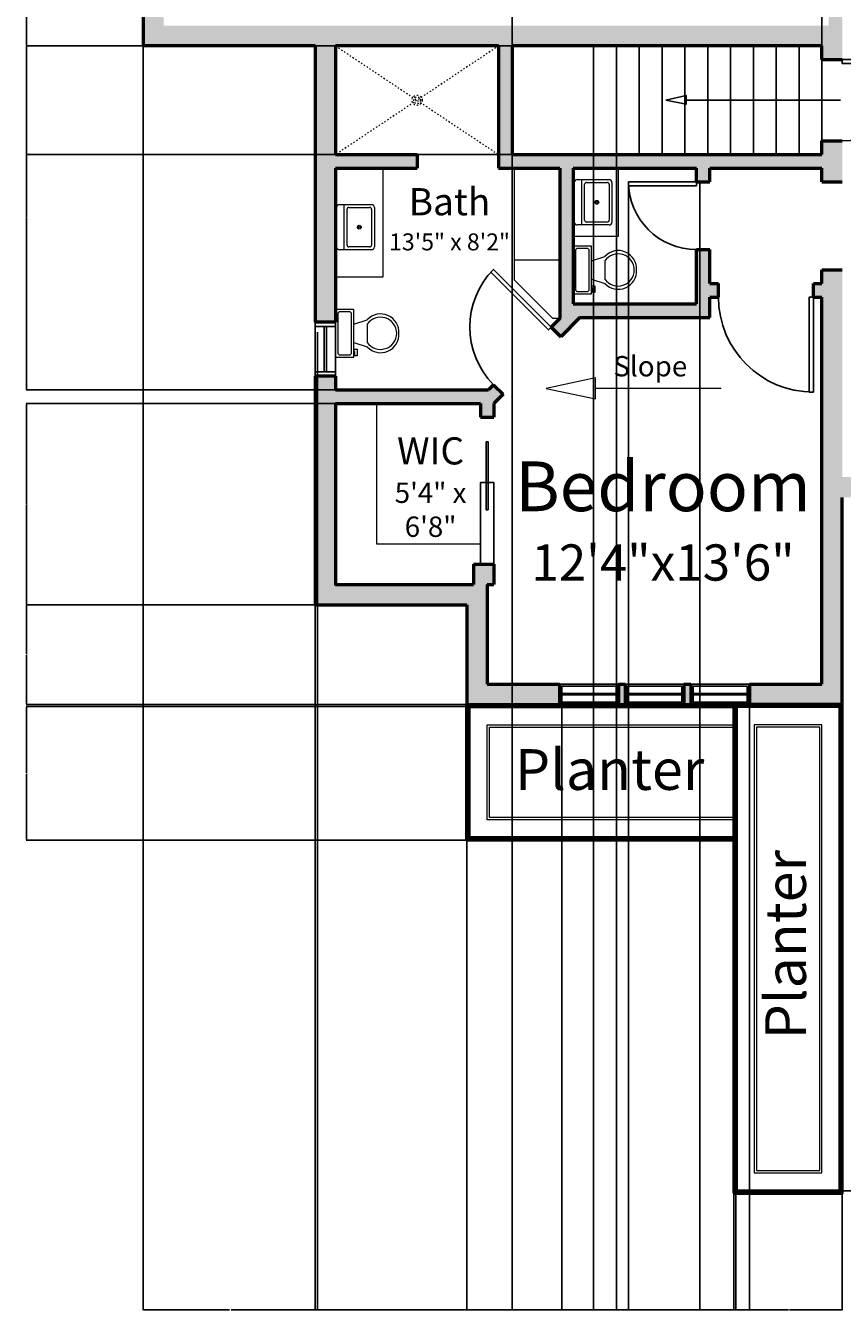
# Model space of a CAD drawing. Units: inches. Extents: x 296 to 2116, y 330 to 1460.
# Tile 1 of 9: x 296 to 657, y 330 to 898. Entities that reach past the tile are written whole.
import ezdxf

# ---------------------------------------------------------------- set-up
doc = ezdxf.new("R2010")
doc.units = ezdxf.units.IN
doc.linetypes.add('ACAD_ISO03W100', pattern=[30, 12, -18])
for name, color, linetype, lineweight in [('A-ANNO-DIMS', 2, 'Continuous', 18), ('A-ANNO-SYMB', 2, 'Continuous', 18), ('A-ANNO-TEXT', 7, 'Continuous', 18), ('A-AREA-IDEN', 7, 'Continuous', 25), ('A-DOOR', 3, 'Continuous', 25), ('A-FLOR-FIXT', 8, 'Continuous', 18), ('A-FLOR-OVHD', 132, 'ACAD_ISO03W100', 18), ('A-FLOR-STRS', 40, 'Continuous', 25), ('A-GLAZ', 4, 'Continuous', 25), ('A-WALL', 7, 'Continuous', 50), ('A-WALL-PATT', 8, 'Continuous', 13), ('L-PLNT', 90, 'Continuous', 18)]:
    doc.layers.add(name, color=color, linetype=linetype, lineweight=lineweight)
doc.styles.add('ATTR', font='romans.shx', dxfattribs={"width": 0.8, "height": 1.075})
doc.styles.get("Standard").update_dxf_attribs({"font": 'arial.ttf'})
doc.dimstyles.get("Standard").update_dxf_attribs({"dimtxt": 0.18, "dimasz": 0.18, "dimexe": 0.18, "dimexo": 0.0625, "dimgap": 0.09, "dimtad": 0, "dimtih": 1, "dimtoh": 1, "dimdec": 4, "dimzin": 0, "dimdsep": 46, "dimtxsty": 'Standard', "dimcen": 0.09, "dimadec": 0, "dimazin": 0, "dimtfac": 1, "dimtdec": 4, "dimtofl": 0, "dimtmove": 0, "dimatfit": 3, "dimfxl": 1, "dimtolj": 1, "dimtzin": 0, "dimarcsym": 0})

# ---------------------------------------------------------------- blocks, each defined once
blk = doc.blocks.new('*U2')
for p, q in [((0, 0), (0, -4)), ((-36, 0), (-36, -4))]:
    blk.add_line(p, q)
blk.add_lwpolyline([(0, 0), (0, 36), (-1.75, 36), (-1.75, 0)], close=True)
blk.add_arc((0, 0), 36, 90, 180)
blk = doc.blocks.new('*U4')
for p, q in [((-30, 0), (-30, -6)), ((0, 0), (0, -6))]:
    blk.add_line(p, q)
blk.add_lwpolyline([(0, 0), (0, 30), (-1.75, 30), (-1.75, 0)], close=True)
blk.add_arc((0, 0), 30, 90, 180)
blk = doc.blocks.new('*U3')
for p, q in [((0, 0), (0, -4)), ((40, 0), (40, -4))]:
    blk.add_line(p, q)
blk.add_lwpolyline([(0, 0), (0, 40), (1.75, 40), (1.75, 0)], close=True)
blk.add_arc((0, 0), 40, 0, 90)
blk = doc.blocks.new('*U15')
for p, q in [((-36, 0), (-36, 6)), ((0, 0), (0, 6))]:
    blk.add_line(p, q)
blk.add_lwpolyline([(0, 0), (0, -36), (-1.75, -36), (-1.75, 0)], close=True)
blk.add_arc((0, 0), 36, 180, 270)
blk = doc.blocks.new('*U29')
for p, q in [((9.5, -6), (9.5, -2)), ((-10, -8.5), (-8, -8.5)), ((-10, -9.5), (-10, -8.5)), ((-7, -9.5), (-10, -9.5)), ((-8, -8.5), (-8, -8)), ((-7, -8), (-7, -9.5)), ((-4, -8), (-6, -14)), ((4, -8), (6, -14)), ((4, -14), (-4, -14))]:
    blk.add_line(p, q)
blk.add_lwpolyline([(10.5, -8), (10.5, 0), (-10.5, 0), (-10.5, -8)], close=True)
for points in [[(-9.5, -2), (-9.5, -6)], [(8.5, -1), (-8.5, -1)], [(-8.5, -7), (8.5, -7)]]:
    blk.add_lwpolyline(points)
for centre, radius, start, end in [((-8.625, -1.875), 0.8839, 81.8699, 188.1301), ((8.625, -1.875), 0.8839, 351.8699, 98.1301), ((-8.625, -6.125), 0.8839, 171.869898, 278.1301), ((8.625, -6.125), 0.8839, 261.8699, 8.1301), ((-0.4772, -19.9188), 8.0953, 133.01722, 273.38), ((0.0374, -19.8731), 7.127, 124.50543, 269.7), ((-0.0373, -19.8731), 7.127, 270.3, 55.4946), ((0.4773, -19.9188), 8.0953, 266.62, 46.9828)]:
    blk.add_arc(centre, radius, start, end)
blk = doc.blocks.new("24'' Sink Single PV")
blk.add_line((-12.00001, -3.999996), (12, -3.999996))
for points in [[(-10.5, 0), (10.5, 0)], [(-12.00001, -18.499996), (-12.00001, -1.5)], [(-10.5, -17.499996), (-10.5, -6.499996)], [(-9.5, -5.499996), (9.5, -5.499996)], [(10.5, -6.499996), (10.5, -17.499996)], [(12, -1.5), (12, -18.499996)], [(10.5, -19.999996), (-10.5, -19.999996)], [(9.5, -18.499996), (-9.5, -18.499996)]]:
    blk.add_lwpolyline(points)
for radius in [1, 0.5]:
    blk.add_circle((0, -11.999996), radius)
for centre, radius, start, end in [((-10.5, -1.5), 1.5, 90, 180), ((-9.5, -6.499996), 1, 90, 180), ((9.5, -6.499996), 1, 0, 90), ((10.5, -1.5), 1.5, 0, 90), ((-10.5, -18.499996), 1.5, 180, 270), ((-9.5, -17.499996), 1, 180, 270), ((9.5, -17.499996), 1, 270, 0), ((10.5, -18.499996), 1.5, 270, 0)]:
    blk.add_arc(centre, radius, start, end)
at = {"style": 'ATTR', "width": 0.8, "flags": 9}
blk.add_attdef('ESTCODE', (0, 0), '', height=0.0048, dxfattribs=at)
blk = doc.blocks.new('SLOPE-ARROW')
blk.add_line((739.99, 662.71), (684.54, 662.71))
blk.add_lwpolyline([(662.67, 662.71), (684.54, 658.1), (684.54, 667.32)], close=True)
blk = doc.blocks.new('*D45')
at = {"layer": 'A-ANNO-DIMS', "color": 0, "lineweight": -2, "transparency": 16777216}
for p, q in [((1156.58, 1407.95), (1235.3, 1407.95)), ((1235.12, 1407.77), (1235.12, 895.66)), ((1235.12, 383.18), (1235.12, 895.29)), ((609.63, 383), (1235.3, 383))]:
    blk.add_line(p, q, dxfattribs=at)
at = {"layer": 'A-ANNO-DIMS', "color": 0, "transparency": 16777216}
for points in [[(1235.09, 1407.77), (1235.15, 1407.77), (1235.12, 1407.95)], [(1235.09, 383.18), (1235.15, 383.18), (1235.12, 383)]]:
    blk.add_solid(points, dxfattribs=at)
at = {"layer": 'Defpoints', "color": 0, "transparency": 16777216}
for p in [(1156.52, 1407.95), (1235.12, 1407.95), (609.57, 383)]:
    blk.add_point(p, dxfattribs=at)
at = {"layer": 'A-ANNO-DIMS', "color": 0, "transparency": 16777216, "insert": (1235.12, 895.48), "char_height": 0.18, "attachment_point": 5}
blk.add_mtext('\\A1;1025', dxfattribs=at)
blk = doc.blocks.new('*D50')
at = {"layer": 'A-ANNO-DIMS', "color": 0, "lineweight": -2, "transparency": 16777216}
for p, q in [((347.52, 888.94), (347.52, 330.22)), ((424.57, 762.44), (424.57, 330.22)), ((347.7, 330.4), (385.65, 330.4)), ((424.39, 330.4), (386.44, 330.4))]:
    blk.add_line(p, q, dxfattribs=at)
at = {"layer": 'A-ANNO-DIMS', "color": 0, "transparency": 16777216}
for points in [[(347.7, 330.43), (347.7, 330.37), (347.52, 330.4)], [(424.39, 330.43), (424.39, 330.37), (424.57, 330.4)]]:
    blk.add_solid(points, dxfattribs=at)
at = {"layer": 'Defpoints', "color": 0, "transparency": 16777216}
for p in [(347.52, 889), (424.57, 762.5), (424.57, 330.4)]:
    blk.add_point(p, dxfattribs=at)
at = {"layer": 'A-ANNO-DIMS', "color": 0, "transparency": 16777216, "insert": (386.05, 330.4), "char_height": 0.18, "attachment_point": 5}
blk.add_mtext('\\A1;77.05', dxfattribs=at)
blk = doc.blocks.new('*D51')
at = {"layer": 'A-ANNO-DIMS', "color": 0, "lineweight": -2, "transparency": 16777216}
for p, q in [((424.57, 762.44), (424.57, 330.22)), ((490.57, 537.98), (490.57, 330.22)), ((424.75, 330.4), (457.35, 330.4)), ((490.39, 330.4), (457.79, 330.4))]:
    blk.add_line(p, q, dxfattribs=at)
at = {"layer": 'A-ANNO-DIMS', "color": 0, "transparency": 16777216}
for points in [[(424.75, 330.43), (424.75, 330.37), (424.57, 330.4)], [(490.39, 330.43), (490.39, 330.37), (490.57, 330.4)]]:
    blk.add_solid(points, dxfattribs=at)
at = {"layer": 'Defpoints', "color": 0, "transparency": 16777216}
for p in [(424.57, 762.5), (490.57, 538.04), (490.57, 330.4)]:
    blk.add_point(p, dxfattribs=at)
at = {"layer": 'A-ANNO-DIMS', "color": 0, "transparency": 16777216, "insert": (457.57, 330.4), "char_height": 0.18, "attachment_point": 5}
blk.add_mtext('\\A1;66', dxfattribs=at)
blk = doc.blocks.new('*D52')
at = {"layer": 'A-ANNO-DIMS', "color": 0, "lineweight": -2, "transparency": 16777216}
for p, q in [((490.57, 537.98), (490.57, 330.22)), ((608.57, 537.98), (608.57, 330.22)), ((490.75, 330.4), (549.29, 330.4)), ((608.39, 330.4), (549.85, 330.4))]:
    blk.add_line(p, q, dxfattribs=at)
at = {"layer": 'A-ANNO-DIMS', "color": 0, "transparency": 16777216}
for points in [[(490.75, 330.43), (490.75, 330.37), (490.57, 330.4)], [(608.39, 330.43), (608.39, 330.37), (608.57, 330.4)]]:
    blk.add_solid(points, dxfattribs=at)
at = {"layer": 'Defpoints', "color": 0, "transparency": 16777216}
for p in [(490.57, 538.04), (608.57, 538.04), (608.57, 330.4)]:
    blk.add_point(p, dxfattribs=at)
at = {"layer": 'A-ANNO-DIMS', "color": 0, "transparency": 16777216, "insert": (549.57, 330.4), "char_height": 0.18, "attachment_point": 5}
blk.add_mtext('\\A1;118', dxfattribs=at)
blk = doc.blocks.new('*D53')
at = {"layer": 'A-ANNO-DIMS', "color": 0, "lineweight": -2, "transparency": 16777216}
for p, q in [((609.57, 382.94), (609.57, 330.22)), ((656.57, 381.94), (656.57, 330.22)), ((609.75, 330.4), (632.85, 330.4)), ((656.39, 330.4), (633.29, 330.4))]:
    blk.add_line(p, q, dxfattribs=at)
at = {"layer": 'A-ANNO-DIMS', "color": 0, "transparency": 16777216}
for points in [[(609.75, 330.43), (609.75, 330.37), (609.57, 330.4)], [(656.39, 330.43), (656.39, 330.37), (656.57, 330.4)]]:
    blk.add_solid(points, dxfattribs=at)
at = {"layer": 'Defpoints', "color": 0, "transparency": 16777216}
for p in [(609.57, 383), (656.57, 382), (656.57, 330.4)]:
    blk.add_point(p, dxfattribs=at)
at = {"layer": 'A-ANNO-DIMS', "color": 0, "transparency": 16777216, "insert": (633.07, 330.4), "char_height": 0.18, "attachment_point": 5}
blk.add_mtext('\\A1;47', dxfattribs=at)
blk = doc.blocks.new('*D57')
at = {"layer": 'A-ANNO-DIMS', "color": 0, "lineweight": -2, "transparency": 16777216}
for p, q in [((491.51, 597), (295.74, 597)), ((295.92, 596.82), (295.92, 567.7)), ((295.92, 538.22), (295.92, 567.34)), ((490.51, 538.04), (295.74, 538.04))]:
    blk.add_line(p, q, dxfattribs=at)
at = {"layer": 'A-ANNO-DIMS', "color": 0, "transparency": 16777216}
for points in [[(295.89, 596.82), (295.95, 596.82), (295.92, 597)], [(295.89, 538.22), (295.95, 538.22), (295.92, 538.04)]]:
    blk.add_solid(points, dxfattribs=at)
at = {"layer": 'Defpoints', "color": 0, "transparency": 16777216}
for p in [(295.92, 597), (491.57, 597), (490.57, 538.04)]:
    blk.add_point(p, dxfattribs=at)
at = {"layer": 'A-ANNO-DIMS', "color": 0, "transparency": 16777216, "insert": (295.92, 567.52), "char_height": 0.18, "attachment_point": 5}
blk.add_mtext('\\A1;58.96', dxfattribs=at)
blk = doc.blocks.new('*D58')
at = {"layer": 'A-ANNO-DIMS', "color": 0, "lineweight": -2, "transparency": 16777216}
for p, q in [((347.46, 1031), (295.74, 1031)), ((295.92, 1030.82), (295.92, 960.18)), ((295.92, 889.18), (295.92, 959.82)), ((347.46, 889), (295.74, 889))]:
    blk.add_line(p, q, dxfattribs=at)
at = {"layer": 'A-ANNO-DIMS', "color": 0, "transparency": 16777216}
for points in [[(295.89, 1030.82), (295.95, 1030.82), (295.92, 1031)], [(295.89, 889.18), (295.95, 889.18), (295.92, 889)]]:
    blk.add_solid(points, dxfattribs=at)
at = {"layer": 'Defpoints', "color": 0, "transparency": 16777216}
for p in [(295.92, 1031), (347.52, 1031), (347.52, 889)]:
    blk.add_point(p, dxfattribs=at)
at = {"layer": 'A-ANNO-DIMS', "color": 0, "transparency": 16777216, "insert": (295.92, 960), "char_height": 0.18, "attachment_point": 5}
blk.add_mtext('\\A1;142', dxfattribs=at)
blk = doc.blocks.new('*D66')
at = {"layer": 'A-ANNO-DIMS', "color": 0, "lineweight": -2, "transparency": 16777216}
for p, q in [((510.57, 889.06), (510.57, 1459.73)), ((510.75, 1459.55), (578.79, 1459.55)), ((647.39, 1459.55), (579.35, 1459.55)), ((647.57, 889.06), (647.57, 1459.73))]:
    blk.add_line(p, q, dxfattribs=at)
at = {"layer": 'A-ANNO-DIMS', "color": 0, "transparency": 16777216}
for points in [[(510.75, 1459.58), (510.75, 1459.52), (510.57, 1459.55)], [(647.39, 1459.58), (647.39, 1459.52), (647.57, 1459.55)]]:
    blk.add_solid(points, dxfattribs=at)
at = {"layer": 'Defpoints', "color": 0, "transparency": 16777216}
for p in [(647.57, 1459.55), (510.57, 889), (647.57, 889)]:
    blk.add_point(p, dxfattribs=at)
at = {"layer": 'A-ANNO-DIMS', "color": 0, "transparency": 16777216, "insert": (579.07, 1459.55), "char_height": 0.18, "attachment_point": 5}
blk.add_mtext('\\A1;137', dxfattribs=at)
blk = doc.blocks.new('*D89')
at = {"layer": 'A-ANNO-DIMS', "color": 0, "lineweight": -2, "transparency": 16777216}
for p, q in [((423.57, 888.94), (423.57, 330.22)), ((510.57, 888.94), (510.57, 330.22)), ((423.75, 330.4), (466.68, 330.4)), ((510.39, 330.4), (467.47, 330.4))]:
    blk.add_line(p, q, dxfattribs=at)
at = {"layer": 'A-ANNO-DIMS', "color": 0, "transparency": 16777216}
for points in [[(423.75, 330.43), (423.75, 330.37), (423.57, 330.4)], [(510.39, 330.43), (510.39, 330.37), (510.57, 330.4)]]:
    blk.add_solid(points, dxfattribs=at)
at = {"layer": 'Defpoints', "color": 0, "transparency": 16777216}
for p in [(423.57, 889), (510.57, 889), (510.57, 330.4)]:
    blk.add_point(p, dxfattribs=at)
at = {"layer": 'A-ANNO-DIMS', "color": 0, "transparency": 16777216, "insert": (467.07, 330.4), "char_height": 0.18, "attachment_point": 5}
blk.add_mtext('\\A1;87.00', dxfattribs=at)
blk = doc.blocks.new('*D90')
at = {"layer": 'A-ANNO-DIMS', "color": 0, "lineweight": -2, "transparency": 16777216}
for p, q in [((546.57, 840.94), (546.57, 330.22)), ((556.67, 840.94), (556.67, 330.22)), ((546.75, 330.4), (551.24, 330.4)), ((556.49, 330.4), (552.01, 330.4))]:
    blk.add_line(p, q, dxfattribs=at)
at = {"layer": 'A-ANNO-DIMS', "color": 0, "transparency": 16777216}
for points in [[(546.75, 330.43), (546.75, 330.37), (546.57, 330.4)], [(556.49, 330.43), (556.49, 330.37), (556.67, 330.4)]]:
    blk.add_solid(points, dxfattribs=at)
at = {"layer": 'Defpoints', "color": 0, "transparency": 16777216}
for p in [(546.57, 841), (556.67, 841), (556.67, 330.4)]:
    blk.add_point(p, dxfattribs=at)
at = {"layer": 'A-ANNO-DIMS', "color": 0, "transparency": 16777216, "insert": (551.62, 330.4), "char_height": 0.18, "attachment_point": 5}
blk.add_mtext('\\A1;10.10', dxfattribs=at)
blk = doc.blocks.new('*D91')
at = {"layer": 'A-ANNO-DIMS', "color": 0, "lineweight": -2, "transparency": 16777216}
for p, q in [((597.01, 889), (295.74, 889)), ((295.92, 888.82), (295.92, 865.18)), ((295.92, 841.18), (295.92, 864.82)), ((597.01, 841), (295.74, 841))]:
    blk.add_line(p, q, dxfattribs=at)
at = {"layer": 'A-ANNO-DIMS', "color": 0, "transparency": 16777216}
for points in [[(295.89, 888.82), (295.95, 888.82), (295.92, 889)], [(295.89, 841.18), (295.95, 841.18), (295.92, 841)]]:
    blk.add_solid(points, dxfattribs=at)
at = {"layer": 'Defpoints', "color": 0, "transparency": 16777216}
for p in [(597.07, 889), (295.92, 841), (597.07, 841)]:
    blk.add_point(p, dxfattribs=at)
at = {"layer": 'A-ANNO-DIMS', "color": 0, "transparency": 16777216, "insert": (295.92, 865), "char_height": 0.18, "attachment_point": 5}
blk.add_mtext('\\A1;48.00', dxfattribs=at)
blk = doc.blocks.new('*D92')
at = {"layer": 'A-ANNO-DIMS', "color": 0, "lineweight": -2, "transparency": 16777216}
for p, q in [((432.51, 731), (295.74, 731)), ((295.92, 730.82), (295.92, 686.68)), ((295.92, 642.18), (295.92, 686.32)), ((423.51, 642), (295.74, 642))]:
    blk.add_line(p, q, dxfattribs=at)
at = {"layer": 'A-ANNO-DIMS', "color": 0, "transparency": 16777216}
for points in [[(295.89, 730.82), (295.95, 730.82), (295.92, 731)], [(295.89, 642.18), (295.95, 642.18), (295.92, 642)]]:
    blk.add_solid(points, dxfattribs=at)
at = {"layer": 'Defpoints', "color": 0, "transparency": 16777216}
for p in [(432.57, 731), (295.92, 642), (423.57, 642)]:
    blk.add_point(p, dxfattribs=at)
at = {"layer": 'A-ANNO-DIMS', "color": 0, "transparency": 16777216, "insert": (295.92, 686.5), "char_height": 0.18, "attachment_point": 5}
blk.add_mtext('\\A1;89.00', dxfattribs=at)
blk = doc.blocks.new('*D93')
at = {"layer": 'A-ANNO-DIMS', "color": 0, "lineweight": -2, "transparency": 16777216}
for p, q in [((423.51, 889), (295.74, 889)), ((295.92, 888.82), (295.92, 813.18)), ((295.92, 737.18), (295.92, 812.82)), ((432.51, 737), (295.74, 737))]:
    blk.add_line(p, q, dxfattribs=at)
at = {"layer": 'A-ANNO-DIMS', "color": 0, "transparency": 16777216}
for points in [[(295.89, 888.82), (295.95, 888.82), (295.92, 889)], [(295.89, 737.18), (295.95, 737.18), (295.92, 737)]]:
    blk.add_solid(points, dxfattribs=at)
at = {"layer": 'Defpoints', "color": 0, "transparency": 16777216}
for p in [(295.92, 889), (423.57, 889), (432.57, 737)]:
    blk.add_point(p, dxfattribs=at)
at = {"layer": 'A-ANNO-DIMS', "color": 0, "transparency": 16777216, "insert": (295.92, 813), "char_height": 0.18, "attachment_point": 5}
blk.add_mtext('\\A1;152.00', dxfattribs=at)
blk = doc.blocks.new('*D94')
at = {"layer": 'A-ANNO-DIMS', "color": 0, "lineweight": -2, "transparency": 16777216}
for p, q in [((423.51, 642), (295.74, 642)), ((295.92, 641.82), (295.92, 620.18)), ((295.92, 598.18), (295.92, 619.82)), ((490.51, 598), (295.74, 598))]:
    blk.add_line(p, q, dxfattribs=at)
at = {"layer": 'A-ANNO-DIMS', "color": 0, "transparency": 16777216}
for points in [[(295.89, 641.82), (295.95, 641.82), (295.92, 642)], [(295.89, 598.18), (295.95, 598.18), (295.92, 598)]]:
    blk.add_solid(points, dxfattribs=at)
at = {"layer": 'Defpoints', "color": 0, "transparency": 16777216}
for p in [(295.92, 642), (423.57, 642), (490.57, 598)]:
    blk.add_point(p, dxfattribs=at)
at = {"layer": 'A-ANNO-DIMS', "color": 0, "transparency": 16777216, "insert": (295.92, 620), "char_height": 0.18, "attachment_point": 5}
blk.add_mtext('\\A1;44.00', dxfattribs=at)
blk = doc.blocks.new('*D102')
at = {"layer": 'A-ANNO-DIMS', "color": 0, "lineweight": -2, "transparency": 16777216}
for p, q in [((562.07, 828.94), (562.07, 330.22)), ((593.59, 828.06), (593.59, 330.22)), ((562.25, 330.4), (577.37, 330.4)), ((593.41, 330.4), (578.29, 330.4))]:
    blk.add_line(p, q, dxfattribs=at)
at = {"layer": 'A-ANNO-DIMS', "color": 0, "transparency": 16777216}
for points in [[(562.25, 330.43), (562.25, 330.37), (562.07, 330.4)], [(593.41, 330.43), (593.41, 330.37), (593.59, 330.4)]]:
    blk.add_solid(points, dxfattribs=at)
at = {"layer": 'Defpoints', "color": 0, "transparency": 16777216}
for p in [(562.07, 829), (593.59, 828.12), (593.59, 330.4)]:
    blk.add_point(p, dxfattribs=at)
at = {"layer": 'A-ANNO-DIMS', "color": 0, "transparency": 16777216, "insert": (577.83, 330.4), "char_height": 0.18, "attachment_point": 5}
blk.add_mtext('\\A1;31.516', dxfattribs=at)
blk = doc.blocks.new('*D105')
at = {"layer": 'A-ANNO-DIMS', "color": 0, "lineweight": -2, "transparency": 16777216}
for p, q in [((532.57, 598.94), (532.57, 330.22)), ((615.57, 597.94), (615.57, 330.22)), ((532.75, 330.4), (573.68, 330.4)), ((615.39, 330.4), (574.47, 330.4))]:
    blk.add_line(p, q, dxfattribs=at)
at = {"layer": 'A-ANNO-DIMS', "color": 0, "transparency": 16777216}
for points in [[(532.75, 330.43), (532.75, 330.37), (532.57, 330.4)], [(615.39, 330.43), (615.39, 330.37), (615.57, 330.4)]]:
    blk.add_solid(points, dxfattribs=at)
at = {"layer": 'Defpoints', "color": 0, "transparency": 16777216}
for p in [(532.57, 599), (615.57, 598), (615.57, 330.4)]:
    blk.add_point(p, dxfattribs=at)
at = {"layer": 'A-ANNO-DIMS', "color": 0, "transparency": 16777216, "insert": (574.07, 330.4), "char_height": 0.18, "attachment_point": 5}
blk.add_mtext('\\A1;83.00', dxfattribs=at)

msp = doc.modelspace()

# ---------------------------------------------------------------- hatches: boundary and pattern name
at = {"layer": 'A-WALL-PATT'}
h = msp.add_hatch(color=256, dxfattribs=at)
h.dxf.hatch_style = 1
h.paths.add_polyline_path([(656.5723, 927.9991), (668.5723, 927.9991), (668.5723, 936.9991), (650.5723, 936.9991), (650.5723, 897.9991), (356.5223, 897.9991), (356.5223, 955.9991), (347.5223, 955.9991), (347.5223, 888.9991), (423.5723, 888.9991), (423.5723, 766.9991), (432.5723, 766.9991), (432.5723, 834.9991), (453.5723, 834.9991), (468.5723, 834.9991), (468.5723, 840.9991), (432.5723, 840.9991), (432.5723, 888.9991), (504.5723, 888.9991), (504.5723, 840.9991), (504.5723, 834.9991), (531.6223, 834.9991), (531.6223, 768.5344), (527.8443, 764.7564), (530.6728, 761.928), (532.087, 760.5138), (540.5723, 768.9991), (598.0723, 768.9991), (598.0723, 777.9991), (601.8223, 777.9991), (601.8223, 782.1991), (601.8223, 783.9991), (598.0723, 783.9991), (598.0723, 798.9991), (592.0723, 798.9991), (592.0723, 774.9991), (537.6223, 774.9991), (537.6223, 834.9991), (592.0723, 834.9991), (592.0723, 828.9991), (598.0723, 828.9991), (598.0723, 834.9991), (647.5723, 834.9991), (647.5723, 828.9991), (656.5723, 828.9991), (656.5723, 846.9991), (650.5723, 846.9991), (647.5723, 846.9991), (647.5723, 840.9991), (510.5723, 840.9991), (510.5723, 888.9991), (647.5723, 888.9991), (647.5723, 882.9991), (656.5723, 882.9991)])
h.paths.add_polyline_path([(432.5723, 730.9991), (496.5723, 730.9991), (496.5723, 724.9991), (502.5723, 724.9991), (502.5723, 730.9991), (506.6311, 735.058), (502.3885, 739.3006), (500.087, 736.9991), (432.5723, 736.9991), (432.5723, 742.9991), (423.5723, 742.9991), (423.5723, 641.9991), (490.5723, 641.9991), (490.5723, 597.9991), (531.5723, 597.9991), (531.5723, 606.9991), (499.5723, 606.9991), (499.5723, 650.9991), (502.5723, 650.9991), (502.5723, 659.9991), (496.5723, 659.9991), (493.5723, 659.9991), (493.5723, 650.9991), (432.5723, 650.9991)])
h.paths.add_polyline_path([(656.5723, 689.4991), (662.5473, 689.4991), (662.5473, 698.4991), (656.5723, 698.4991), (656.5723, 789.9991), (647.5723, 789.9991), (647.5723, 783.9991), (643.8223, 783.9991), (643.8223, 777.9991), (647.5723, 777.9991), (647.5723, 606.9991), (615.5723, 606.9991), (615.5723, 597.9991), (656.5723, 597.9991)])
h.paths.add_polyline_path([(761.5223, 780.9541), (797.5223, 780.9541), (797.5223, 789.9541), (761.5223, 789.9541), (761.5223, 858.9541), (797.5223, 858.9541), (797.5223, 867.9541), (752.5223, 867.9541), (752.5223, 698.4991), (746.5473, 698.4991), (746.5473, 694.2991), (746.5473, 689.4991), (752.5223, 689.4991), (752.5223, 624.9541), (761.5223, 624.9541)])
h.paths.add_polyline_path([(1102.5223, 795.9541), (1093.5223, 795.9541), (1093.5223, 789.9541), (1063.5223, 789.9541), (881.5223, 789.9541), (881.5223, 837.9541), (911.5223, 837.9541), (911.5223, 849.9541), (907.5223, 849.9541), (905.5223, 849.9541), (905.5223, 843.9541), (845.5223, 843.9541), (845.5223, 834.9541), (849.0223, 834.9541), (851.5223, 834.9541), (851.5223, 837.9541), (875.5223, 837.9541), (875.5223, 789.9541), (851.5223, 789.9541), (851.5223, 792.9541), (845.5223, 792.9541), (845.5223, 789.9541), (833.5223, 789.9541), (833.5223, 785.1541), (833.5223, 780.9541), (1049.5223, 780.9541), (1049.5223, 726.9541), (1053.7223, 726.9541), (1058.5223, 726.9541), (1058.5223, 780.9541), (1102.5223, 780.9541)])
h.paths.add_polyline_path([(761.5223, 588.9541), (752.5223, 588.9541), (752.5223, 564.9541), (761.5223, 564.9541)])
h.paths.add_polyline_path([(809.5223, 480.9541), (761.5223, 480.9541), (761.5223, 528.9541), (752.5223, 528.9541), (752.5223, 471.9541), (809.5223, 471.9541)])
h.paths.add_polyline_path([(1058.5223, 684.9541), (1049.5223, 684.9541), (1049.5223, 480.9541), (1001.5223, 480.9541), (1001.5223, 476.4541), (1001.5223, 471.9541), (1058.5223, 471.9541)])
h.paths.add_polyline_path([(794.5223, 1013.9991), (800.5223, 1013.9991), (800.5223, 1019.9991), (794.5223, 1019.9991), (794.5223, 1296.9541), (785.5223, 1296.9541), (785.5223, 1221.9991), (752.5223, 1221.9991), (752.5223, 1212.9991), (788.5223, 1212.9991), (788.5223, 936.9991), (752.5223, 936.9991), (752.5223, 927.9991), (794.5223, 927.9991)])
h.paths.add_polyline_path([(450.0223, 1191.9991), (398.5223, 1191.9991), (398.5223, 1137.9991), (407.5223, 1137.9991), (407.5223, 1182.9991), (450.0223, 1182.9991)])
h.paths.add_polyline_path([(576.5223, 1212.9991), (612.5223, 1212.9991), (612.5223, 1221.9991), (567.5223, 1221.9991), (567.5223, 1191.9991), (540.0223, 1191.9991), (540.0223, 1182.9991), (576.5223, 1182.9991)])
h.paths.add_polyline_path([(407.5223, 1060.9991), (398.5223, 1060.9991), (398.5223, 1030.9991), (392.5223, 1030.9991), (392.5223, 1021.9991), (407.5223, 1021.9991)])
h.paths.add_polyline_path([(356.5223, 1030.9991), (347.5223, 1030.9991), (347.5223, 1015.9991), (356.5223, 1015.9991), (356.5223, 1021.9991)])
h.paths.add_polyline_path([(788.5223, 1129.9991), (770.0334, 1131.3572, 0.43585667), (767.8869, 1129.3626), (767.8869, 1108.3618, 0.31855172), (769.8942, 1105.5308), (788.5223, 1098.9991)], flags=17)
h.paths.add_polyline_path([(788.5223, 1050.9991), (769.8942, 1044.4674, 0.31855172), (767.8869, 1041.6364), (767.8869, 1020.6356, 0.43585667), (770.0334, 1018.641), (788.5223, 1019.9991)], flags=17)
h.paths.add_polyline_path([(893.5223, 1066.9541), (851.5223, 1066.9541), (851.5223, 1069.9541), (845.5223, 1069.9541), (845.5223, 1019.9991), (839.5223, 1019.9991), (839.5223, 1013.9991), (845.5223, 1013.9991), (845.5223, 891.9541), (863.5223, 891.9541), (863.5223, 897.9541), (851.5223, 897.9541), (851.5223, 927.9541), (905.5223, 927.9541), (905.5223, 897.9541), (893.5223, 897.9541), (893.5223, 891.9541), (905.5223, 891.9541), (905.5223, 885.9541), (911.5223, 885.9541), (911.5223, 927.9541), (1030.5223, 927.9541), (1030.5223, 936.9541), (1013.5223, 936.9541), (1013.5223, 996.9541), (1093.5223, 996.9541), (1093.5223, 936.9541), (1066.5223, 936.9541), (1066.5223, 927.9541), (1093.5223, 927.9541), (1093.5223, 921.9541), (1102.5223, 921.9541), (1102.5223, 1013.9541), (1093.5223, 1013.9541), (1093.5223, 1002.9541), (1013.5223, 1002.9541), (1013.5223, 1060.9541), (1013.5223, 1066.9541), (1007.5223, 1066.9541), (1007.5223, 1042.9541), (977.5223, 1042.9541), (977.5223, 1066.9541), (965.5223, 1066.9541), (965.5223, 1060.9541), (971.5223, 1060.9541), (971.5223, 1036.9541), (1007.5223, 1036.9541), (1007.5223, 936.9541), (851.5223, 936.9541), (851.5223, 1060.9541), (893.5223, 1060.9541)])
h.paths.add_polyline_path([(851.5223, 1150.9541), (919.5223, 1150.9541), (919.5223, 1114.9541), (911.5223, 1114.9541), (911.5223, 1108.9541), (925.5223, 1108.9541), (925.5223, 1150.9541), (1007.5223, 1150.9541), (1007.5223, 1114.9541), (1013.5223, 1114.9541), (1013.5223, 1150.9541), (1046.5223, 1150.9541), (1046.5223, 1159.9541), (1007.5223, 1159.9541), (1007.5223, 1186.9541), (998.5223, 1186.9541), (998.5223, 1156.9541), (845.5223, 1156.9541), (845.5223, 1105.9541), (851.5223, 1105.9541)])
h.paths.add_polyline_path([(1102.5223, 1156.9541), (1102.5223, 1159.9541), (1088.5223, 1159.9541), (1088.5223, 1150.9541), (1093.5223, 1150.9541), (1093.5223, 1147.9541), (1102.5223, 1147.9541)])
h.paths.add_polyline_path([(1102.5223, 1111.9541), (1093.5223, 1111.9541), (1093.5223, 1066.9541), (1047.5223, 1066.9541), (1047.5223, 1030.9541), (1053.5223, 1030.9541), (1053.5223, 1060.9541), (1093.5223, 1060.9541), (1093.5223, 1049.9541), (1102.5223, 1049.9541)])
h.paths.add_polyline_path([(1102.5223, 837.9541), (1093.5223, 837.9541), (1093.5223, 831.9541), (1102.5223, 831.9541)], flags=17)
h.paths.add_polyline_path([(1102.5223, 879.9541), (1093.5223, 879.9541), (1093.5223, 873.9541), (1102.5223, 873.9541)])
h.paths.add_polyline_path([(839.5223, 1353.9541), (785.5223, 1353.9541), (785.5223, 1338.9541), (794.5223, 1338.9541), (794.5223, 1344.9541), (839.5223, 1344.9541)])
h.paths.add_polyline_path([(1007.5223, 1353.9541), (953.5223, 1353.9541), (953.5223, 1344.9541), (998.5223, 1344.9541), (998.5223, 1314.9541), (1007.5223, 1314.9541)])
h.paths.add_polyline_path([(917.5223, 1353.9541), (914.5223, 1353.9541), (914.5223, 1344.9541), (917.5223, 1344.9541)])
h.paths.add_polyline_path([(878.5223, 1353.9541), (875.5223, 1353.9541), (875.5223, 1344.9541), (878.5223, 1344.9541)])
h.paths.add_polyline_path([(1007.5223, 1278.9541), (998.5223, 1278.9541), (998.5223, 1222.9541), (1007.5223, 1222.9541)])
h.paths.add_polyline_path([(407.5223, 1101.9991), (398.5223, 1101.9991), (398.5223, 1096.9991), (407.5223, 1096.9991)])
h.paths.add_polyline_path([(560.5723, 606.9991), (557.5723, 606.9991), (557.5723, 597.9991), (560.5723, 597.9991)])
h.paths.add_polyline_path([(589.5723, 606.9991), (586.5723, 606.9991), (586.5723, 597.9991), (589.5723, 597.9991)])

# ---------------------------------------------------------------- linework, layer by layer
at = {"layer": 'A-DOOR'}
for points in [[(500.0723, 683.9991), (500.0723, 713.9991), (499.0723, 713.9991), (499.0723, 683.9991)], [(496.5723, 659.9991), (496.5723, 695.9991), (502.5723, 695.9991), (502.5723, 659.9991)]]:
    msp.add_lwpolyline(points, close=True, dxfattribs=at)
at = {"layer": 'A-FLOR-FIXT'}
for p, q in [((511.6517, 785.5049), (511.6517, 834.9991)), ((557.6223, 804.9991), (557.6223, 834.9991)), ((537.6223, 804.9991), (557.6223, 804.9991)), ((511.6517, 794.5049), (531.6223, 794.5049)), ((528.6223, 768.5344), (511.6517, 785.5049)), ((531.6223, 768.5344), (528.6223, 768.5344))]:
    msp.add_line(p, q, dxfattribs=at)
msp.add_lwpolyline([(432.5723, 786.9991), (453.5723, 786.9991), (453.5723, 834.9991), (432.5723, 834.9991)], close=True, dxfattribs=at)
msp.add_lwpolyline([(450.5723, 730.9991), (450.5723, 668.9991), (496.5723, 668.9991), (496.5723, 659.9991)], dxfattribs=at)
at = {"layer": 'A-FLOR-OVHD', "ltscale": 0.05}
for p, q in [((432.5723, 888.9991), (504.5723, 840.9991)), ((504.5723, 888.9991), (432.5723, 840.9991))]:
    msp.add_line(p, q, dxfattribs=at)
msp.add_lwpolyline([(504.5723, 888.9991), (432.5723, 888.9991), (432.5723, 840.9991), (504.5723, 840.9991)], close=True, dxfattribs=at)
for radius in [2.25, 1.5]:
    msp.add_circle((468.5723, 864.9991), radius, dxfattribs=at)
at = {"layer": 'A-FLOR-STRS'}
for p, q in [((546.5723, 888.9991), (546.5723, 840.9991)), ((556.6723, 888.9991), (556.6723, 840.9991)), ((566.7723, 888.9991), (566.7723, 840.9991)), ((576.8723, 888.9991), (576.8723, 840.9991)), ((586.9723, 888.9991), (586.9723, 840.9991)), ((597.0723, 888.9991), (597.0723, 840.9991)), ((607.1723, 888.9991), (607.1723, 840.9991)), ((617.2723, 888.9991), (617.2723, 840.9991)), ((627.3723, 888.9991), (627.3723, 840.9991)), ((637.4723, 888.9991), (637.4723, 840.9991)), ((647.5723, 888.9991), (647.5723, 840.9991))]:
    msp.add_line(p, q, dxfattribs=at)
msp.add_lwpolyline([(578.6155, 864.9991), (587.4834, 867.1441), (587.4834, 863.2509)], close=True, dxfattribs=at)
msp.add_lwpolyline([(655.824, 864.9991), (587.4834, 864.9991)], dxfattribs=at)
at = {"layer": 'A-GLAZ'}
for p, q in [((423.5723, 764.9991), (432.5723, 764.9991)), ((427.5723, 744.9991), (427.5723, 764.9991)), ((428.5723, 764.9991), (428.5723, 744.9991)), ((432.5723, 744.9991), (423.5723, 744.9991)), ((532.5723, 602.7491), (556.5723, 602.7491)), ((532.5723, 602.2491), (556.5723, 602.2491)), ((561.5723, 602.7491), (585.5723, 602.7491)), ((561.5723, 602.2491), (585.5723, 602.2491)), ((590.5723, 602.7491), (614.5723, 602.7491)), ((590.5723, 602.2491), (614.5723, 602.2491))]:
    msp.add_line(p, q, dxfattribs=at)
for points in [[(432.5723, 766.9991), (432.5723, 742.9991), (423.5723, 742.9991), (423.5723, 766.9991)], [(531.5723, 606.9991), (557.5723, 606.9991), (557.5723, 597.9991), (531.5723, 597.9991)], [(532.5723, 605.9991), (556.5723, 605.9991), (556.5723, 598.9991), (532.5723, 598.9991)], [(560.5723, 606.9991), (586.5723, 606.9991), (586.5723, 597.9991), (560.5723, 597.9991)], [(561.5723, 605.9991), (585.5723, 605.9991), (585.5723, 598.9991), (561.5723, 598.9991)], [(589.5723, 606.9991), (615.5723, 606.9991), (615.5723, 597.9991), (589.5723, 597.9991)], [(590.5723, 605.9991), (614.5723, 605.9991), (614.5723, 598.9991), (590.5723, 598.9991)]]:
    msp.add_lwpolyline(points, close=True, dxfattribs=at)
at = {"layer": 'A-WALL'}
for p, q in [((347.5223, 955.9991), (347.5223, 888.9991)), ((423.5723, 888.9991), (347.5223, 888.9991)), ((423.5723, 888.9991), (423.5723, 766.9991)), ((432.5723, 888.9991), (432.5723, 840.9991)), ((504.5723, 888.9991), (432.5723, 888.9991)), ((504.5723, 888.9991), (504.5723, 834.9991)), ((647.5723, 888.9991), (510.5723, 888.9991)), ((510.5723, 888.9991), (510.5723, 840.9991)), ((647.5723, 882.9991), (647.5723, 888.9991)), ((647.5723, 882.9991), (656.5723, 882.9991)), ((647.5723, 840.9991), (647.5723, 846.9991)), ((647.5723, 846.9991), (656.5723, 846.9991)), ((432.5723, 840.9991), (468.5723, 840.9991)), ((468.5723, 840.9991), (468.5723, 834.9991)), ((510.5723, 840.9991), (647.5723, 840.9991)), ((432.5723, 834.9991), (432.5723, 766.9991)), ((432.5723, 834.9991), (468.5723, 834.9991)), ((504.5723, 834.9991), (531.6223, 834.9991)), ((531.6223, 834.9991), (531.6223, 768.5344)), ((537.6223, 834.9991), (537.6223, 774.9991)), ((537.6223, 834.9991), (592.0723, 834.9991)), ((592.0723, 828.9991), (592.0723, 834.9991)), ((598.0723, 828.9991), (598.0723, 834.9991)), ((598.0723, 834.9991), (647.5723, 834.9991)), ((647.5723, 828.9991), (647.5723, 834.9991)), ((592.0723, 828.9991), (598.0723, 828.9991)), ((647.5723, 828.9991), (656.5723, 828.9991)), ((592.0723, 774.9991), (592.0723, 798.9991)), ((592.0723, 798.9991), (598.0723, 798.9991)), ((598.0723, 783.9991), (598.0723, 798.9991)), ((647.5723, 783.9991), (647.5723, 789.9991)), ((647.5723, 789.9991), (656.5723, 789.9991)), ((598.0723, 783.9991), (601.8223, 783.9991)), ((601.8223, 777.9991), (601.8223, 783.9991)), ((643.8223, 777.9991), (643.8223, 783.9991)), ((643.8223, 783.9991), (647.5723, 783.9991)), ((598.0723, 768.9991), (598.0723, 777.9991)), ((598.0723, 777.9991), (601.8223, 777.9991)), ((643.8223, 777.9991), (647.5723, 777.9991)), ((647.5723, 606.9991), (647.5723, 777.9991)), ((537.6223, 774.9991), (592.0723, 774.9991)), ((432.5723, 766.9991), (423.5723, 766.9991)), ((531.6223, 768.5344), (527.8443, 764.7564)), ((540.5723, 768.9991), (532.087, 760.5138)), ((540.5723, 768.9991), (598.0723, 768.9991)), ((527.8443, 764.7564), (532.087, 760.5138)), ((432.5723, 742.9991), (423.5723, 742.9991)), ((423.5723, 742.9991), (423.5723, 641.9991)), ((432.5723, 742.9991), (432.5723, 736.9991)), ((502.3885, 739.3006), (500.087, 736.9991)), ((502.3885, 739.3006), (506.6311, 735.058)), ((432.5723, 736.9991), (500.087, 736.9991)), ((506.6311, 735.058), (502.5723, 730.9991)), ((432.5723, 730.9991), (496.5723, 730.9991)), ((496.5723, 730.9991), (496.5723, 724.9991)), ((502.5723, 730.9991), (502.5723, 724.9991)), ((496.5723, 724.9991), (502.5723, 724.9991)), ((656.5723, 597.9991), (656.5723, 689.4991)), ((493.5723, 659.9991), (502.5723, 659.9991)), ((493.5723, 659.9991), (493.5723, 650.9991)), ((502.5723, 659.9991), (502.5723, 650.9991)), ((499.5723, 650.9991), (499.5723, 606.9991)), ((499.5723, 650.9991), (502.5723, 650.9991)), ((423.5723, 641.9991), (490.5723, 641.9991)), ((490.5723, 641.9991), (490.5723, 597.9991)), ((499.5723, 606.9991), (531.5723, 606.9991)), ((531.5723, 606.9991), (531.5723, 597.9991)), ((557.5723, 606.9991), (557.5723, 597.9991)), ((557.5723, 606.9991), (560.5723, 606.9991)), ((560.5723, 606.9991), (560.5723, 597.9991)), ((586.5723, 606.9991), (586.5723, 597.9991)), ((586.5723, 606.9991), (589.5723, 606.9991)), ((589.5723, 606.9991), (589.5723, 597.9991)), ((615.5723, 606.9991), (615.5723, 597.9991)), ((615.5723, 606.9991), (647.5723, 606.9991)), ((490.5723, 597.9991), (531.5723, 597.9991)), ((557.5723, 597.9991), (560.5723, 597.9991)), ((586.5723, 597.9991), (589.5723, 597.9991)), ((615.5723, 597.9991), (656.5723, 597.9991))]:
    msp.add_line(p, q, dxfattribs=at)
for points in [[(432.5723, 730.9991), (432.5723, 650.9991), (493.5723, 650.9991)], [(608.5723, 538.0399), (490.5723, 538.0399), (490.5723, 597.9991), (608.5723, 597.9991)], [(608.5723, 539.0399), (491.5723, 539.0399), (491.5723, 596.9991), (608.5723, 596.9991)]]:
    msp.add_lwpolyline(points, dxfattribs=at)
for points in [[(608.5723, 381.9991), (656.5723, 381.9991), (656.5723, 597.9991), (608.5723, 597.9991)], [(609.5723, 382.9991), (655.5723, 382.9991), (655.5723, 596.9991), (609.5723, 596.9991)]]:
    msp.add_lwpolyline(points, close=True, dxfattribs=at)
at = {"layer": 'L-PLNT'}
for points in [[(608.5723, 547.0399), (499.5723, 547.0399), (499.5723, 588.9991), (608.5723, 588.9991)], [(608.5723, 548.0399), (500.5723, 548.0399), (500.5723, 587.9991), (608.5723, 587.9991)]]:
    msp.add_lwpolyline(points, dxfattribs=at)
for points in [[(617.5723, 390.9991), (647.5723, 390.9991), (647.5723, 588.9991), (617.5723, 588.9991)], [(618.5723, 391.9991), (646.5723, 391.9991), (646.5723, 587.9991), (618.5723, 587.9991)]]:
    msp.add_lwpolyline(points, close=True, dxfattribs=at)

# ---------------------------------------------------------------- block references
at = {"layer": 'A-ANNO-SYMB'}
msp.add_blockref('SLOPE-ARROW', (-137.0397, 74.9696), dxfattribs=at)
at = {"layer": 'A-DOOR'}
for name, p, rotation in [('*U15', (656.5723, 882.9991), 90.00000000000003), ('*U4', (592.0723, 828.9991), 90.00000000000003), ('*U2', (527.8443, 764.7564), 44.99999999999957)]:
    msp.add_blockref(name, p, dxfattribs=dict(at, rotation=rotation))
at = {"layer": 'A-DOOR', "xscale": 1.05, "yscale": 1.05, "zscale": 1.05, "rotation": 180}
msp.add_blockref('*U3', (643.8223, 777.9991), dxfattribs=at)
at = {"layer": 'A-FLOR-FIXT', "xscale": 0.8333413357028808, "yscale": 0.8333413357028808, "zscale": 0.8333413357028808, "rotation": 90}
for p in [(538.0778, 819.9148), (433.0278, 808.9213)]:
    msp.add_blockref("24'' Sink Single PV", p, dxfattribs=at)
at = {"layer": 'A-FLOR-FIXT', "rotation": 90}
for p in [(537.6223, 789.9991), (432.5723, 761.9991)]:
    msp.add_blockref('*U29', p, dxfattribs=at)

# ---------------------------------------------------------------- texts
at = {"layer": 'A-ANNO-TEXT', "insert": (550.6943, 751.9684), "char_height": 9, "attachment_point": 1}
msp.add_mtext_dynamic_manual_height_columns('\\pxqc;Slope', width=41.969454, gutter_width=12.5, heights=[0], dxfattribs=at)
at = {"layer": 'A-AREA-IDEN', "attachment_point": 1}
for s, width, insert, char_height in [('\\pxqc;Bath\\P{\\H0.625x;13\'5" x 8\'2"}', 53.982916, (455.9255, 826.159), 12), ('\\pxqc;WIC\\P{\\H0.75x;5\'4" x 6\'8"}', 49.048889, (450.0234, 716.0413), 12), ('\\pxqc;{\\fArial|b1|i0|c0|p34;\\H0.91667x;Bedroom\\H1.09091x;\\P\\fArial|b0|i0|c0|p34;\\H0.66667x;12\'4"x13\'6"}', 167.942646, (493.3182, 705.3849), 24), ('\\pxqc;{\\fArial|b1|i0|c0|p34;\\H0.75x;Planter}', 82.300549, (512.5519, 578.2161), 24)]:
    msp.add_mtext_dynamic_manual_height_columns(s, width=width, gutter_width=12.5, heights=[0], dxfattribs=dict(at, insert=insert, char_height=char_height))
at = {"layer": 'A-AREA-IDEN', "insert": (622.5006, 442.4184), "char_height": 24, "attachment_point": 1, "rotation": 90}
msp.add_mtext_dynamic_manual_height_columns('\\pxqc;{\\fArial|b1|i0|c0|p34;\\H0.75x;Planter}', width=98.796099, gutter_width=12.5, heights=[0], dxfattribs=at)

# ---------------------------------------------------------------- dimensions: what is measured, and where the dimension line sits
at = {"layer": 'A-ANNO-DIMS'}
for base, p1, p2, override, picture, middle in [((647.5723, 1459.5541), (510.5723, 888.9991), (647.5723, 888.9991), {"dimdec": 0, "dimlfac": 1, "dimrnd": 0, "dimzin": 0, "dimdsep": 46, "dimlunit": 2}, '*D66', (579.0723, 1459.5541)), ((424.5723, 330.3991), (347.5223, 888.9991), (424.5723, 762.4991), {"dimdec": 2, "dimlfac": 1, "dimrnd": 0, "dimzin": 0, "dimdsep": 46, "dimlunit": 2}, '*D50', (386.0473, 330.3991)), ((510.5723, 330.3991), (423.5723, 888.9991), (510.5723, 888.9991), {"dimdec": 2, "dimlfac": 1, "dimrnd": 0, "dimzin": 0, "dimdsep": 46, "dimlunit": 2}, '*D89', (467.0723, 330.3991)), ((556.6723, 330.3991), (546.5723, 840.9991), (556.6723, 840.9991), {"dimdec": 2, "dimlfac": 1, "dimrnd": 0, "dimzin": 0, "dimdsep": 46, "dimlunit": 2}, '*D90', (551.6223, 330.3991)), ((593.58781, 330.39909), (562.07227, 828.99909), (593.58781, 828.12409), {"dimdec": 3, "dimlfac": 1, "dimrnd": 0, "dimzin": 0, "dimdsep": 46, "dimlunit": 2}, '*D102', (577.83004, 330.39909)), ((490.5723, 330.3991), (424.5723, 762.4991), (490.5723, 538.0399), {"dimdec": 0, "dimlfac": 1, "dimrnd": 0, "dimzin": 0, "dimdsep": 46, "dimlunit": 2}, '*D51', (457.5723, 330.3991)), ((615.5723, 330.3991), (532.5723, 598.9991), (615.5723, 597.9991), {"dimdec": 2, "dimlfac": 1, "dimrnd": 0, "dimzin": 0, "dimdsep": 46, "dimlunit": 2}, '*D105', (574.0723, 330.3991)), ((608.5723, 330.3991), (490.5723, 538.0399), (608.5723, 538.0399), {"dimdec": 0, "dimlfac": 1, "dimrnd": 0, "dimzin": 0, "dimdsep": 46, "dimlunit": 2}, '*D52', (549.5723, 330.3991)), ((656.5723, 330.3991), (609.5723, 382.9991), (656.5723, 381.9991), {"dimdec": 0, "dimlfac": 1, "dimrnd": 0, "dimzin": 0, "dimdsep": 46, "dimlunit": 2}, '*D53', (633.0723, 330.3991))]:
    dim = msp.add_linear_dim(base=base, p1=p1, p2=p2, dimstyle='Standard', override=override, dxfattribs=at)
    dim.commit()
    dim.dimension.update_dxf_attribs({"geometry": picture, "text_midpoint": middle})
for base, p1, p2, override, picture, middle in [((1235.1223, 1407.9541), (609.5723, 382.9991), (1156.5223, 1407.9541), {"dimdec": 0, "dimlfac": 1, "dimrnd": 0, "dimzin": 0, "dimdsep": 46, "dimlunit": 2}, '*D45', (1235.1223, 895.4766)), ((295.9223, 1030.9991), (347.5223, 888.9991), (347.5223, 1030.9991), {"dimdec": 0, "dimlfac": 1, "dimrnd": 0, "dimzin": 0, "dimdsep": 46, "dimlunit": 2}, '*D58', (295.9223, 959.9991)), ((295.9223, 888.9991), (432.5723, 736.9991), (423.5723, 888.9991), {"dimdec": 2, "dimlfac": 1, "dimrnd": 0, "dimzin": 0, "dimdsep": 46, "dimlunit": 2}, '*D93', (295.9223, 812.9991)), ((295.9223, 840.9991), (597.0723, 888.9991), (597.0723, 840.9991), {"dimdec": 2, "dimlfac": 1, "dimrnd": 0, "dimzin": 0, "dimdsep": 46, "dimlunit": 2}, '*D91', (295.9223, 864.9991)), ((295.9223, 641.9991), (432.5723, 730.9991), (423.5723, 641.9991), {"dimdec": 2, "dimlfac": 1, "dimrnd": 0, "dimzin": 0, "dimdsep": 46, "dimlunit": 2}, '*D92', (295.9223, 686.4991)), ((295.9223, 641.9991), (490.5723, 597.9991), (423.5723, 641.9991), {"dimdec": 2, "dimlfac": 1, "dimrnd": 0, "dimzin": 0, "dimdsep": 46, "dimlunit": 2}, '*D94', (295.9223, 619.9991)), ((295.9223, 596.9991), (490.5723, 538.0399), (491.5723, 596.9991), {"dimdec": 2, "dimlfac": 1, "dimrnd": 0, "dimzin": 0, "dimdsep": 46, "dimlunit": 2}, '*D57', (295.9223, 567.5195))]:
    dim = msp.add_linear_dim(base=base, p1=p1, p2=p2, angle=90, dimstyle='Standard', override=override, dxfattribs=at)
    dim.commit()
    dim.dimension.update_dxf_attribs({"geometry": picture, "text_midpoint": middle})

doc.saveas('drawing.dxf')
